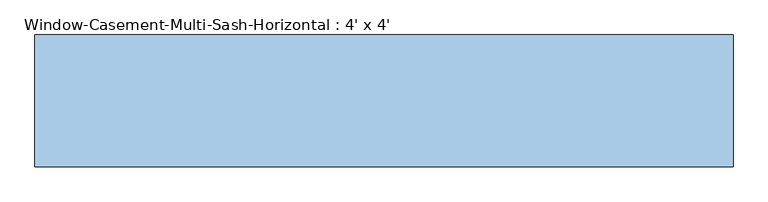
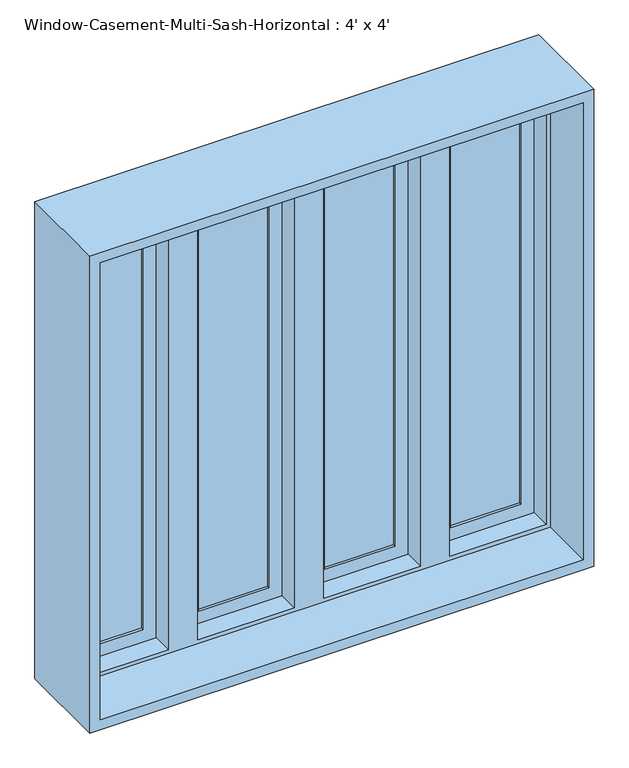
"""IFC4 building model written with IfcOpenShell, lengths in millimetres: window geometry, Window-Casement-Multi-Sash-Horizontal : 4' x 4'."""

from ifc_helpers import new_model, si_unit, frame, origin, place, context, project, spatial, polyline, outline, extrude, faceted_brep, source, transform, mapped, element, save


def window_casement_multi_sash_horizontal_4_x_4_8de01852(model_context):
    return source(origin(), model_context, "Body", "SolidModel", [
        extrude(outline(polyline([(2108.2, 330.2), (939.8, 330.2), (939.8, 584.2), (2108.2, 584.2), (2108.2, 330.2)]), holes=[polyline([(2066.3296875, 542.3296875), (981.6703125, 542.3296875), (981.6703125, 372.0703125), (2066.3296875, 372.0703125), (2066.3296875, 542.3296875)])]), frame((0.0, 73.725, 0.0), z_axis=(0.0, 1.0, 0.0), x_axis=(0.0, 0.0, 1.0)), (0.0, 0.0, 1.0), 31.75),
        extrude(outline(polyline([(2108.2, -584.2), (939.8, -584.2), (939.8, -330.2), (2108.2, -330.2), (2108.2, -584.2)]), holes=[polyline([(2066.3296875, -372.0703125), (981.6703125, -372.0703125), (981.6703125, -542.3296875), (2066.3296875, -542.3296875), (2066.3296875, -372.0703125)])]), frame((0.0, 73.725, 0.0), z_axis=(0.0, 1.0, 0.0), x_axis=(0.0, 0.0, 1.0)), (0.0, 0.0, 1.0), 31.75),
        extrude(outline(polyline([(-372.0703125, 99.125), (-372.0703125, 92.775), (-542.3296875, 92.775), (-542.3296875, 99.125), (-372.0703125, 99.125)])), frame((0.0, 0.0, 981.6703125), z_axis=(0.0, 0.0, 1.0), x_axis=(1.0, 0.0, 0.0)), (0.0, 0.0, 1.0), 1084.659375),
        extrude(outline(polyline([(-372.0703125, 86.425), (-372.0703125, 80.075), (-542.3296875, 80.075), (-542.3296875, 86.425), (-372.0703125, 86.425)])), frame((0.0, 0.0, 981.6703125), z_axis=(0.0, 0.0, 1.0), x_axis=(1.0, 0.0, 0.0)), (0.0, 0.0, 1.0), 1084.659375),
        extrude(outline(polyline([(542.3296875, 99.125), (542.3296875, 92.775), (372.0703125, 92.775), (372.0703125, 99.125), (542.3296875, 99.125)])), frame((0.0, 0.0, 981.6703125), z_axis=(0.0, 0.0, 1.0), x_axis=(1.0, 0.0, 0.0)), (0.0, 0.0, 1.0), 1084.659375),
        extrude(outline(polyline([(542.3296875, 86.425), (542.3296875, 80.075), (372.0703125, 80.075), (372.0703125, 86.425), (542.3296875, 86.425)])), frame((0.0, 0.0, 981.6703125), z_axis=(0.0, 0.0, 1.0), x_axis=(1.0, 0.0, 0.0)), (0.0, 0.0, 1.0), 1084.659375),
        extrude(outline(polyline([(-67.2703125, 99.125), (-67.2703125, 92.775), (-237.5296875, 92.775), (-237.5296875, 99.125), (-67.2703125, 99.125)])), frame((0.0, 0.0, 981.6703125), z_axis=(0.0, 0.0, 1.0), x_axis=(1.0, 0.0, 0.0)), (0.0, 0.0, 1.0), 1084.659375),
        extrude(outline(polyline([(-67.2703125, 86.425), (-67.2703125, 80.075), (-237.5296875, 80.075), (-237.5296875, 86.425), (-67.2703125, 86.425)])), frame((0.0, 0.0, 981.6703125), z_axis=(0.0, 0.0, 1.0), x_axis=(1.0, 0.0, 0.0)), (0.0, 0.0, 1.0), 1084.659375),
        extrude(outline(polyline([(237.5296875, 99.125), (237.5296875, 92.775), (67.2703125, 92.775), (67.2703125, 99.125), (237.5296875, 99.125)])), frame((0.0, 0.0, 981.6703125), z_axis=(0.0, 0.0, 1.0), x_axis=(1.0, 0.0, 0.0)), (0.0, 0.0, 1.0), 1084.659375),
        extrude(outline(polyline([(237.5296875, 86.425), (237.5296875, 80.075), (67.2703125, 80.075), (67.2703125, 86.425), (237.5296875, 86.425)])), frame((0.0, 0.0, 981.6703125), z_axis=(0.0, 0.0, 1.0), x_axis=(1.0, 0.0, 0.0)), (0.0, 0.0, 1.0), 1084.659375),
        faceted_brep([(-330.2, 73.725, 2108.2), (-584.2, 73.725, 2108.2), (-584.2, 115.0, 2108.2), (584.2, 115.0, 2108.2), (584.2, 73.725, 2108.2), (330.2, 73.725, 2108.2), (330.2, 111.825, 2108.2), (279.4, 111.825, 2108.2), (279.4, 73.725, 2108.2), (25.4, 73.725, 2108.2), (25.4, 111.825, 2108.2), (-25.4, 111.825, 2108.2), (-25.4, 73.725, 2108.2), (-279.4, 73.725, 2108.2), (-279.4, 111.825, 2108.2), (-330.2, 111.825, 2108.2), (-574.0796875, 22.925, 2098.0796875), (-574.0796875, 73.725, 2098.0796875), (-340.3203125, 73.725, 2098.0796875), (-340.3203125, 22.925, 2098.0796875), (574.0796875, 73.725, 2098.0796875), (574.0796875, 22.925, 2098.0796875), (340.3203125, 22.925, 2098.0796875), (340.3203125, 73.725, 2098.0796875), (-269.2796875, 73.725, 2098.0796875), (-35.5203125, 73.725, 2098.0796875), (-35.5203125, 22.925, 2098.0796875), (-269.2796875, 22.925, 2098.0796875), (35.5203125, 73.725, 2098.0796875), (269.2796875, 73.725, 2098.0796875), (269.2796875, 22.925, 2098.0796875), (35.5203125, 22.925, 2098.0796875), (-584.2, -115.0, 2108.2), (-584.2, 22.925, 2108.2), (584.2, 22.925, 2108.2), (584.2, -115.0, 2108.2), (-609.6, 115.0, 2133.6), (-609.6, -115.0, 2133.6), (609.6, -115.0, 2133.6), (609.6, 115.0, 2133.6), (584.2, 115.0, 939.8), (584.2, 73.725, 939.8), (574.0796875, 73.725, 949.9203125), (574.0796875, 22.925, 949.9203125), (584.2, 22.925, 939.8), (584.2, -115.0, 939.8), (609.6, -115.0, 914.4), (609.6, 115.0, 914.4), (330.2, 73.725, 939.8), (-584.2, 115.0, 939.8), (-584.2, 73.725, 939.8), (-330.2, 73.725, 939.8), (-330.2, 111.825, 939.8), (-279.4, 111.825, 939.8), (-279.4, 73.725, 939.8), (-25.4, 73.725, 939.8), (-25.4, 111.825, 939.8), (25.4, 111.825, 939.8), (25.4, 73.725, 939.8), (279.4, 73.725, 939.8), (279.4, 111.825, 939.8), (330.2, 111.825, 939.8), (340.3203125, 73.725, 949.9203125), (340.3203125, 22.925, 949.9203125), (-574.0796875, 73.725, 949.9203125), (-574.0796875, 22.925, 949.9203125), (-340.3203125, 22.925, 949.9203125), (-340.3203125, 73.725, 949.9203125), (-35.5203125, 73.725, 949.9203125), (-269.2796875, 73.725, 949.9203125), (-269.2796875, 22.925, 949.9203125), (-35.5203125, 22.925, 949.9203125), (269.2796875, 73.725, 949.9203125), (35.5203125, 73.725, 949.9203125), (35.5203125, 22.925, 949.9203125), (269.2796875, 22.925, 949.9203125), (-584.2, 22.925, 939.8), (-584.2, -115.0, 939.8), (-609.6, -115.0, 914.4), (-609.6, 115.0, 914.4)], [[[0, 1, 2, 3, 4, 5, 6, 7, 8, 9, 10, 11, 12, 13, 14, 15]], [[16, 17, 18, 19]], [[20, 21, 22, 23]], [[24, 25, 26, 27]], [[28, 29, 30, 31]], [[32, 33, 34, 35]], [[36, 37, 38, 39]], [[4, 3, 40, 41]], [[21, 20, 42, 43]], [[35, 34, 44, 45]], [[39, 38, 46, 47]], [[48, 41, 40, 49, 50, 51, 52, 53, 54, 55, 56, 57, 58, 59, 60, 61]], [[43, 42, 62, 63]], [[64, 65, 66, 67]], [[68, 69, 70, 71]], [[72, 73, 74, 75]], [[45, 44, 76, 77]], [[47, 46, 78, 79]], [[2, 1, 50, 49]], [[4, 41, 48, 5], [20, 23, 62, 42]], [[50, 1, 0, 51], [64, 67, 18, 17]], [[12, 55, 54, 13], [69, 68, 25, 24]], [[8, 59, 58, 9], [73, 72, 29, 28]], [[17, 16, 65, 64]], [[44, 34, 33, 76], [16, 19, 66, 65], [27, 26, 71, 70], [31, 30, 75, 74], [21, 43, 63, 22]], [[33, 32, 77, 76]], [[38, 37, 78, 46], [32, 35, 45, 77]], [[37, 36, 79, 78]], [[36, 39, 47, 79], [3, 2, 49, 40]], [[18, 67, 66, 19]], [[69, 24, 27, 70]], [[53, 14, 13, 54]], [[14, 53, 52, 15]], [[15, 52, 51, 0]], [[25, 68, 71, 26]], [[73, 28, 31, 74]], [[57, 10, 9, 58]], [[10, 57, 56, 11]], [[11, 56, 55, 12]], [[6, 61, 60, 7]], [[7, 60, 59, 8]], [[29, 72, 75, 30]], [[62, 23, 22, 63]], [[61, 6, 5, 48]]]),
        extrude(outline(polyline([(2108.2, 25.4), (939.8, 25.4), (939.8, 279.4), (2108.2, 279.4), (2108.2, 25.4)]), holes=[polyline([(2066.3296875, 237.5296875), (981.6703125, 237.5296875), (981.6703125, 67.2703125), (2066.3296875, 67.2703125), (2066.3296875, 237.5296875)])]), frame((0.0, 73.725, 0.0), z_axis=(0.0, 1.0, 0.0), x_axis=(0.0, 0.0, 1.0)), (0.0, 0.0, 1.0), 31.75),
        extrude(outline(polyline([(2108.2, -279.4), (939.8, -279.4), (939.8, -25.4), (2108.2, -25.4), (2108.2, -279.4)]), holes=[polyline([(2066.3296875, -67.2703125), (981.6703125, -67.2703125), (981.6703125, -237.5296875), (2066.3296875, -237.5296875), (2066.3296875, -67.2703125)])]), frame((0.0, 73.725, 0.0), z_axis=(0.0, 1.0, 0.0), x_axis=(0.0, 0.0, 1.0)), (0.0, 0.0, 1.0), 31.75),
    ])


if __name__ == "__main__":
    model = new_model("IFC4")
    model_context = context("Model", 3, world=origin())
    ifc_project = project(units=[si_unit("LENGTHUNIT", "METRE", prefix="MILLI")], contexts=[model_context])
    site = spatial("IfcSite", under=ifc_project)
    building = spatial("IfcBuilding", under=site)
    placement = place(None, origin())
    window_casement_multi_sash_horizontal_4_x_4_shape = window_casement_multi_sash_horizontal_4_x_4_8de01852(model_context)
    element("IfcWindow", 1, ObjectType="Window-Casement-Multi-Sash-Horizontal : 4' x 4'", at=placement, inside=building, context=model_context, shape_type="MappedRepresentation", body=[
        mapped(window_casement_multi_sash_horizontal_4_x_4_shape, transform((0.0, 0.0, 0.0), x_axis=(1.0, 0.0, 0.0), y_axis=(0.0, 1.0, 0.0), z_axis=(0.0, 0.0, 1.0))),
    ])
    save(model, "model.ifc")

# Revit data of these elements
# Type "Window-Casement-Multi-Sash-Horizontal : 4' x 4'"
#   Type Mark = "W1"
#   Fire Rating = "0.5h"
#   Assembly Code = "B2020100"
#   Analytic Construction = "Double glazing - domestic"
#   Window Inset [instance default] = 0' - 0 5/8"
#   Wall Thickness [instance default] = 0' - 6"
#   Visual Light Transmittance = 0.81
#   Thermal Resistance (R) = 1.8146 (h·ft²·°F)/BTU
#   Solar Heat Gain Coefficient = 0.76
#   Rough Width = 4' - 0 1/2"
#   Rough Height = 4' - 0 1/2"
#   Open Window Width = 1' - 0"
#   Heat Transfer Coefficient (U) = 0.5511 BTU/(h·ft²·°F)
#   Height = 4' - 0"
#   Frame Gap 3 [instance default] = 0' - 1 83/128"
#   Frame Gap 2 [instance default] = 0' - 0 5/8"
#   Frame Gap 1 = 0' - 1 51/128"
#   Default Sill Height = 3' - 0"
#   Width = 4' - 0"
#   Frame Material = Metal - Aluminum
#   Glass Panel Material = Glass
#   Wall Closure = (empty or 0)
# Element 1 (IfcWindow, "Window-Casement-Multi-Sash-Horizontal : 4' x 4'")
#   Wall Thickness = 0' - 9.05512"
#   Materials on its faces: "Metal - Aluminum", "Glass"
# Materials
#   "Metal - Aluminum": class "Metal", colour RGB 247 247 247, transparency 0
#   "Glass": class "Glass", colour RGB 0 128 192, transparency 0.75, Description = "Soda Lime Glass", Cost = 0
